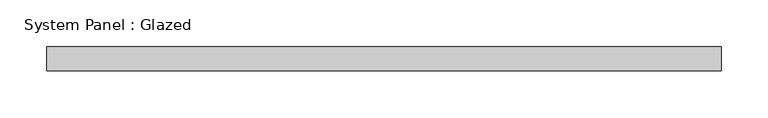
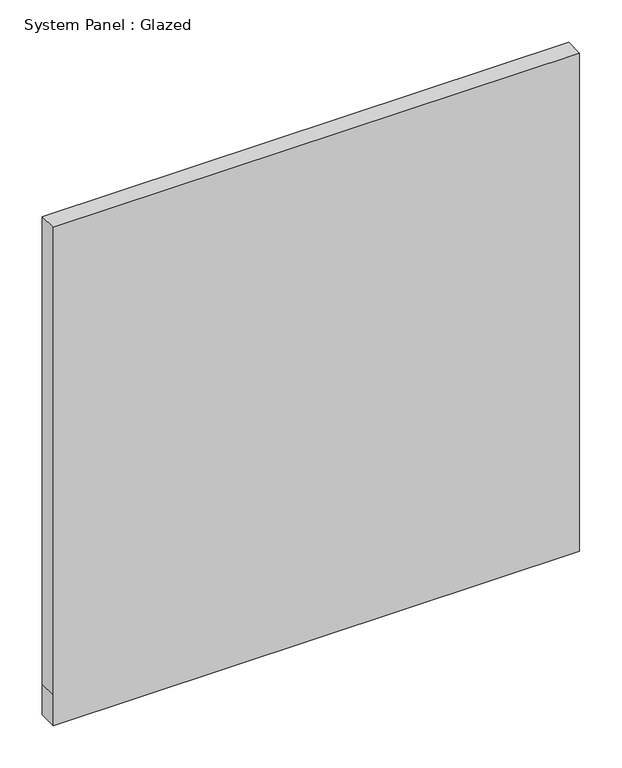
"""IFC4 building model written with IfcOpenShell, lengths in millimetres: plate geometry, System Panel : Glazed."""

from ifc_helpers import new_model, si_unit, frame, origin, place, context, project, spatial, polyline, outline, extrude, source, transform, mapped, element, save


def system_panel_glazed_64ba1ee3(model_context):
    return source(origin(), model_context, "Body", "SweptSolid", [
        extrude(outline(polyline([(0.0, -358.775), (0.0, 358.775), (44.45, 358.775), (717.55, 358.775), (717.55, -358.775), (44.45, -358.775), (0.0, -358.775)])), frame((0.0, 19.05, 0.0), z_axis=(0.0, 1.0, 0.0), x_axis=(0.0, 0.0, 1.0)), (0.0, 0.0, 1.0), 25.4),
    ])


if __name__ == "__main__":
    model = new_model("IFC4")
    model_context = context("Model", 3, world=origin())
    ifc_project = project(units=[si_unit("LENGTHUNIT", "METRE", prefix="MILLI")], contexts=[model_context])
    site = spatial("IfcSite", under=ifc_project)
    building = spatial("IfcBuilding", under=site)
    placement = place(None, origin())
    system_panel_glazed_shape = system_panel_glazed_64ba1ee3(model_context)
    element("IfcPlate", 1, ObjectType="System Panel : Glazed", at=placement, inside=building, context=model_context, shape_type="MappedRepresentation", body=[
        mapped(system_panel_glazed_shape, transform((0.0, 0.0, 0.0), x_axis=(1.0, 0.0, 0.0), y_axis=(0.0, 1.0, 0.0), z_axis=(0.0, 0.0, 1.0))),
    ])
    save(model, "model.ifc")

# Revit data of these elements
# Type "System Panel : Glazed"
#   Construction Type Id = "GSP4R"
#   Analytic Construction = "1/8 in Pilkington single glazing"
#   Visual Light Transmittance = 0.9
#   Solar Heat Gain Coefficient = 0.86
#   Heat Transfer Coefficient (U) = 1.18115 BTU/(h·ft²·°F)
#   Define Thermal Properties by = 1
# Element 1 (IfcPlate, "System Panel : Glazed")
#   Materials on its faces: "Glass"
# Materials
#   "Glass": class "Glass", colour RGB 0 128 192, transparency 0.75, Description = "Soda Lime Glass", Cost = 0
